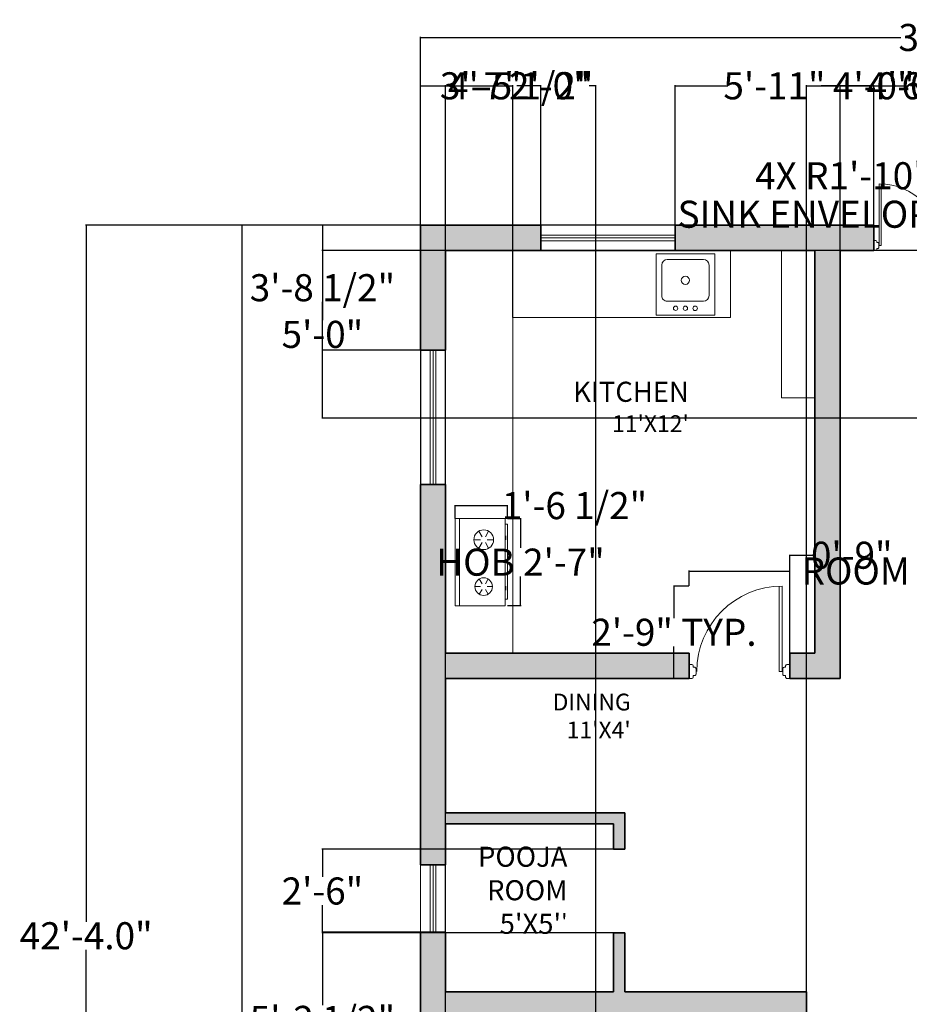
# Model space of a CAD drawing. Units: inches. Extents: x 2103 to 2702, y 2405 to 3142.
# Tile 3 of 7: x 2103 to 2421, y 2790 to 3142. Entities that reach past the tile are written whole.
import ezdxf

# ---------------------------------------------------------------- set-up
doc = ezdxf.new("R2010")
doc.units = ezdxf.units.IN
doc.linetypes.add('0', pattern=[0])
for name, color, linetype, lineweight in [('00 FURNITURE', 15, 'Continuous', 15), ('A-ANNO-DIMS', 2, 'Continuous', 18), ('A-AREA-IDEN', 7, 'Continuous', 18), ('A-EQPM', 9, 'Continuous', 18), ('A-FLOR-CASE', 8, 'Continuous', 18), ('A-FLOR-FIXT', 9, 'Continuous', 18), ('A-WALL-PATT', 8, 'Continuous', 9), ('A_TEXT_SMALL', 18, 'Continuous', 5), ('doors', 4, 'Continuous', 18), ('WALL', 7, 'Continuous', 35), ('WINDOW', 160, '0', 5), ('windows', 4, 'Continuous', 18)]:
    doc.layers.add(name, color=color, linetype=linetype, lineweight=lineweight)
doc.layers.add('FURN3D', color=229, linetype='Continuous', lineweight=5, true_color=0x4a3f41)
doc.layers.add('furniture', color=34, linetype='Continuous')
doc.styles.get("Standard").update_dxf_attribs({"font": 'arial.ttf'})
doc.dimstyles.get("Standard").update_dxf_attribs({"dimtxt": 9.68, "dimasz": 0.18, "dimexe": 0.18, "dimexo": 0.0625, "dimgap": 0.09, "dimtad": 0, "dimtih": 1, "dimtoh": 1, "dimdec": 1, "dimzin": 0, "dimdsep": 46, "dimlunit": 3, "dimtxsty": 'Standard', "dimcen": 0.09, "dimadec": 0, "dimazin": 0, "dimtfac": 1, "dimtdec": 1, "dimtofl": 0, "dimtmove": 0, "dimatfit": 3, "dimfxl": 1, "dimtolj": 1, "dimtzin": 0, "dimarcsym": 0})

# ---------------------------------------------------------------- blocks, each defined once
blk = doc.blocks.new('DDD')
at = {"layer": '00 FURNITURE'}
for p, q in [((-12579.77, -15859.53), (-12579.77, -15829.05)), ((-12578.77, -15859.53), (-12578.77, -15829.03)), ((-12612.02, -15857.03), (-12612.02, -15862.03)), ((-12611.02, -15857.03), (-12612.02, -15857.03)), ((-12610.52, -15858.03), (-12610.52, -15857.53)), ((-12577.52, -15858.03), (-12577.52, -15857.53)), ((-12577.02, -15857.03), (-12576.02, -15857.03)), ((-12576.02, -15857.03), (-12576.02, -15862.03)), ((-12610.52, -15861.53), (-12610.52, -15861.03)), ((-12578.77, -15859.53), (-12579.77, -15859.53)), ((-12577.52, -15861.53), (-12577.52, -15861.03)), ((-12612.02, -15862.03), (-12611.02, -15862.03)), ((-12576.02, -15862.03), (-12577.02, -15862.03))]:
    blk.add_line(p, q, dxfattribs=at)
for points in [[(-12610.52, -15861.03), (-12610.02, -15861.03, 0.414214), (-12609.52, -15860.53), (-12609.52, -15858.53, 0.414214), (-12610.02, -15858.03), (-12610.52, -15858.03)], [(-12577.52, -15861.03), (-12578.02, -15861.03, -0.414214), (-12578.52, -15860.53), (-12578.52, -15858.53, -0.414214), (-12578.02, -15858.03), (-12577.52, -15858.03)]]:
    blk.add_lwpolyline(points, format="xyb", dxfattribs=at)
for centre, radius, start, end in [((-12578.77, -15859.53), 30.5, 90, 180), ((-12611.02, -15857.53), 0.5, 0, 90), ((-12577.02, -15857.53), 0.5, 90, 180), ((-12611.02, -15861.53), 0.5, 270, 0), ((-12577.02, -15861.53), 0.5, 180, 270)]:
    blk.add_arc(centre, radius, start, end, dxfattribs=at)
blk = doc.blocks.new('PUJA')
at = {"layer": '00 FURNITURE'}
for p, q in [((-1941.8, -16091.75), (-1938.89, -16091.75)), ((-1941.8, -16092.33), (-1941.8, -16091.75)), ((-1941.22, -16092.62), (-1941.51, -16092.62)), ((-1939.18, -16092.62), (-1939.47, -16092.62)), ((-1938.89, -16091.75), (-1938.89, -16092.33)), ((-1940.35, -16093.35), (-1958.14, -16093.35)), ((-1940.35, -16093.93), (-1958.13, -16093.93)), ((-1940.35, -16093.35), (-1940.35, -16093.93)), ((-1940.35, -16128.93), (-1958.14, -16128.93)), ((-1940.35, -16128.35), (-1958.13, -16128.35)), ((-1941.8, -16129.96), (-1941.8, -16130.54)), ((-1941.22, -16129.66), (-1941.51, -16129.66)), ((-1940.35, -16128.93), (-1940.35, -16128.35)), ((-1939.18, -16129.66), (-1939.47, -16129.66)), ((-1938.89, -16130.54), (-1938.89, -16129.96)), ((-1941.8, -16130.54), (-1938.89, -16130.54))]:
    blk.add_line(p, q, dxfattribs=at)
for points in [[(-1939.47, -16092.62), (-1939.47, -16092.91, -0.414214), (-1939.76, -16093.21), (-1940.93, -16093.21, -0.414214), (-1941.22, -16092.91), (-1941.22, -16092.62)], [(-1939.47, -16129.66), (-1939.47, -16129.37, 0.414214), (-1939.76, -16129.08), (-1940.93, -16129.08, 0.414214), (-1941.22, -16129.37), (-1941.22, -16129.66)]]:
    blk.add_lwpolyline(points, format="xyb", dxfattribs=at)
for centre, radius, start, end in [((-1941.51, -16092.33), 0.292, 180, 270), ((-1939.18, -16092.33), 0.292, 270, 0), ((-1940.35, -16093.35), 17.79, 180, 270), ((-1940.35, -16128.93), 17.79, 90, 180), ((-1941.51, -16129.96), 0.292, 90, 180), ((-1939.18, -16129.96), 0.292, 0, 90)]:
    blk.add_arc(centre, radius, start, end, dxfattribs=at)
blk = doc.blocks.new('window')
at = {"layer": 'furniture'}
for p, q in [((1745.13, 2764.08), (1745.13, 2716.08)), ((1754.13, 2716.08), (1754.13, 2764.08))]:
    blk.add_line(p, q, dxfattribs=at)
at = {"layer": 'WINDOW'}
for p, q in [((1748.63, 2764.08), (1748.63, 2716.08)), ((1749.63, 2764.08), (1749.63, 2716.08)), ((1750.63, 2764.08), (1750.63, 2716.08))]:
    blk.add_line(p, q, dxfattribs=at)
blk = doc.blocks.new('ventilator')
at = {"layer": 'windows'}
for p, q in [((1922.12, 2523.05), (1898.12, 2523.05)), ((1922.12, 2522.05), (1898.12, 2522.05)), ((1922.12, 2521.05), (1898.12, 2521.05))]:
    blk.add_line(p, q, dxfattribs=at)
blk.add_lwpolyline([(1898.12, 2526.55), (1898.12, 2517.55), (1922.12, 2517.55), (1922.12, 2526.55)], close=True, dxfattribs=at)
blk = doc.blocks.new('A$C21540130')
at = {"layer": 'FURN3D'}
for p, q in [((1.57, 0), (1.57, 31.11)), ((9.61, 25.31), (8.63, 27.01)), ((10.79, 25.31), (11.77, 27.01)), ((9.02, 24.29, -27.54), (7.06, 24.29, -27.54)), ((9.61, 23.27), (8.63, 21.57)), ((10.79, 23.27), (11.77, 21.57)), ((11.38, 24.29, -27.54), (13.34, 24.29, -27.54)), ((9.61, 8.56), (8.43, 10.6)), ((10.79, 8.56), (11.97, 10.6)), ((9.02, 7.54), (6.67, 7.54)), ((11.38, 7.54), (13.73, 7.54)), ((9.61, 6.52), (8.43, 4.48)), ((10.79, 6.52), (11.97, 4.48))]:
    blk.add_line(p, q, dxfattribs=at)
for points in [[(0, 0), (0, 31.11), (17.9, 31.11), (17.9, 0)], [(18.68, 1.96), (18.68, 28.83), (17.9, 28.83), (17.9, 1.96)]]:
    blk.add_lwpolyline(points, close=True, dxfattribs=at)
for centre, radius in [((10.2, 24.29), 3.14), ((10.2, 7.54), 3.53)]:
    blk.add_circle(centre, radius, dxfattribs=at)
for points in [[(17.9, 24.03), (18.29, 24.03), (17.9, 25.6), (18.29, 25.6)], [(17.9, 6.05), (18.29, 6.05), (17.9, 7.62), (18.29, 7.62)]]:
    blk.add_solid(points, dxfattribs=at)
blk = doc.blocks.new('reh-flat-2')
at = {"layer": 'A_TEXT_SMALL'}
for p, q in [((486053827.2, -394630231.2), (486054182.4, -394629799.8)), ((486054182.4, -394629799.8), (486054596.6, -394630140.9)), ((486053979.5, -394630126.3), (486054157.1, -394629910.6)), ((486054228.6, -394629903.6), (486054483.5, -394630113.5)), ((486054596.6, -394630140.9), (486054241.4, -394630572.3)), ((486054241.4, -394630572.3), (486053827.2, -394630231.2)), ((486054241.3, -394630407.7), (486053986.4, -394630197.8)), ((486054490.4, -394630185), (486054312.8, -394630400.7))]:
    blk.add_line(p, q, dxfattribs=at)
for centre, radius in [((486054234.9, -394630155.7), 38.1), ((486054004.1, -394630296.2), 20.1), ((486054072.7, -394630352.7), 20.1), ((486054141.4, -394630409.3), 20.1)]:
    blk.add_circle(centre, radius, dxfattribs=at)
for centre, start, end in [((486054196.3, -394629942.9), 50.53053, 140.53053), ((486054018.7, -394630158.5), 140.53053, 230.53053), ((486054451.2, -394630152.8), 320.53053, 50.53053), ((486054273.6, -394630368.4), 230.53053, 320.53053)]:
    blk.add_arc(centre, 50.8, start, end, dxfattribs=at)
blk = doc.blocks.new('*D15')
at = {"layer": 'A-ANNO-DIMS', "color": 0, "lineweight": -2, "transparency": 16777216}
for p, q in [((2246.43, 3068.91), (2246.43, 3136.18)), ((2246.61, 3136), (2418.13, 3136)), ((2606.25, 3136), (2434.73, 3136)), ((2606.43, 3068.91), (2606.43, 3136.18))]:
    blk.add_line(p, q, dxfattribs=at)
at = {"layer": 'A-ANNO-DIMS', "color": 0, "transparency": 16777216}
for points in [[(2246.61, 3136.03), (2246.61, 3135.97), (2246.43, 3136)], [(2606.25, 3136.03), (2606.25, 3135.97), (2606.43, 3136)]]:
    blk.add_solid(points, dxfattribs=at)
at = {"layer": 'Defpoints', "color": 0, "transparency": 16777216}
for p in [(2606.43, 3136), (2246.43, 3068.85), (2606.43, 3068.85)]:
    blk.add_point(p, dxfattribs=at)
at = {"layer": 'A-ANNO-DIMS', "color": 0, "transparency": 16777216, "insert": (2426.43, 3136), "char_height": 9.68, "attachment_point": 5}
blk.add_mtext("\\A1;30'", dxfattribs=at)
blk = doc.blocks.new('*D16')
at = {"layer": 'A-ANNO-DIMS', "color": 0, "lineweight": -2, "transparency": 16777216}
for p, q in [((2246.37, 3068.85), (2182.44, 3068.85)), ((2182.62, 3068.67), (2182.62, 2762.88)), ((2182.62, 2447.03), (2182.62, 2752.81)), ((2246.37, 2446.85), (2182.44, 2446.85))]:
    blk.add_line(p, q, dxfattribs=at)
at = {"layer": 'A-ANNO-DIMS', "color": 0, "transparency": 16777216}
for points in [[(2182.59, 3068.67), (2182.65, 3068.67), (2182.62, 3068.85)], [(2182.59, 2447.03), (2182.65, 2447.03), (2182.62, 2446.85)]]:
    blk.add_solid(points, dxfattribs=at)
at = {"layer": 'Defpoints', "color": 0, "transparency": 16777216}
for p in [(2246.43, 3068.85), (2182.62, 2446.85), (2246.43, 2446.85)]:
    blk.add_point(p, dxfattribs=at)
at = {"layer": 'A-ANNO-DIMS', "color": 0, "transparency": 16777216, "insert": (2182.62, 2757.85), "char_height": 9.68, "attachment_point": 5}
blk.add_mtext('\\A1;51\'-10.0"', dxfattribs=at)
blk = doc.blocks.new('*D17')
at = {"layer": 'A-ANNO-DIMS', "color": 0, "lineweight": -2, "transparency": 16777216}
for p, q in [((2246.37, 3068.85), (2126.76, 3068.85)), ((2126.94, 3068.67), (2126.94, 2819.88)), ((2126.94, 2561.03), (2126.94, 2809.81)), ((2246.37, 2560.85), (2126.76, 2560.85))]:
    blk.add_line(p, q, dxfattribs=at)
at = {"layer": 'A-ANNO-DIMS', "color": 0, "transparency": 16777216}
for points in [[(2126.91, 3068.67), (2126.97, 3068.67), (2126.94, 3068.85)], [(2126.91, 2561.03), (2126.97, 2561.03), (2126.94, 2560.85)]]:
    blk.add_solid(points, dxfattribs=at)
at = {"layer": 'Defpoints', "color": 0, "transparency": 16777216}
for p in [(2246.43, 3068.85), (2126.94, 2560.85), (2246.43, 2560.85)]:
    blk.add_point(p, dxfattribs=at)
at = {"layer": 'A-ANNO-DIMS', "color": 0, "transparency": 16777216, "insert": (2126.94, 2814.85), "char_height": 9.68, "attachment_point": 5}
blk.add_mtext('\\A1;42\'-4.0"', dxfattribs=at)
blk = doc.blocks.new('*D22')
at = {"layer": 'A-ANNO-DIMS', "color": 0, "lineweight": -2, "transparency": 16777216}
for p, q in [((2342.43, 2939.91), (2342.43, 2945.43)), ((2342.61, 2945.25), (2378.25, 2945.25)), ((2378.43, 2939.91), (2378.43, 2945.43)), ((2378.43, 2945.25), (2378.61, 2945.25))]:
    blk.add_line(p, q, dxfattribs=at)
at = {"layer": 'A-ANNO-DIMS', "color": 0, "transparency": 16777216}
for points in [[(2342.61, 2945.28), (2342.61, 2945.22), (2342.43, 2945.25)], [(2378.25, 2945.28), (2378.25, 2945.22), (2378.43, 2945.25)]]:
    blk.add_solid(points, dxfattribs=at)
at = {"layer": 'Defpoints', "color": 0, "transparency": 16777216}
for p in [(2378.43, 2945.25), (2342.43, 2939.85), (2378.43, 2939.85)]:
    blk.add_point(p, dxfattribs=at)
at = {"layer": 'A-ANNO-DIMS', "color": 0, "transparency": 16777216, "insert": (2453.03, 2945.25), "char_height": 9.68, "attachment_point": 5}
blk.add_mtext('\\A1;ROOM DOOR 3\'-0" TYP.', dxfattribs=at)
blk = doc.blocks.new('*D23')
at = {"layer": 'A-ANNO-DIMS', "color": 0, "lineweight": -2, "transparency": 16777216}
for p, q in [((2342.37, 2939.85), (2336.85, 2939.85)), ((2337.03, 2939.67), (2337.03, 2928.38)), ((2337.03, 2907.03), (2337.03, 2918.31)), ((2342.37, 2906.85), (2336.85, 2906.85))]:
    blk.add_line(p, q, dxfattribs=at)
at = {"layer": 'A-ANNO-DIMS', "color": 0, "transparency": 16777216}
for points in [[(2337, 2939.67), (2337.06, 2939.67), (2337.03, 2939.85)], [(2337, 2907.03), (2337.06, 2907.03), (2337.03, 2906.85)]]:
    blk.add_solid(points, dxfattribs=at)
at = {"layer": 'Defpoints', "color": 0, "transparency": 16777216}
for p in [(2337.03, 2939.85), (2342.43, 2939.85), (2342.43, 2906.85)]:
    blk.add_point(p, dxfattribs=at)
at = {"layer": 'A-ANNO-DIMS', "color": 0, "transparency": 16777216, "insert": (2337.03, 2923.35), "char_height": 9.68, "attachment_point": 5}
blk.add_mtext('\\A1;2\'-9" TYP.', dxfattribs=at)
blk = doc.blocks.new('*D32')
at = {"layer": 'A-ANNO-DIMS', "color": 0, "lineweight": -2, "transparency": 16777216}
for p, q in [((2523.7, 3069.82), (2527.3, 3072.78)), ((2527.05, 3072.8), (2526.87, 3072.8)), ((2527.16, 3072.66), (2527.05, 3072.8)), ((2546.29, 3049.43), (2527.27, 3072.52)), ((2542.95, 3046.44), (2546.55, 3049.4))]:
    blk.add_line(p, q, dxfattribs=at)
at = {"layer": 'A-ANNO-DIMS', "color": 0, "transparency": 16777216}
for points in [[(2527.3, 3072.54), (2527.25, 3072.51), (2527.16, 3072.66)], [(2546.31, 3049.45), (2546.27, 3049.41), (2546.41, 3049.29)]]:
    blk.add_solid(points, dxfattribs=at)
at = {"layer": 'Defpoints', "color": 0, "transparency": 16777216}
for p in [(2523.65, 3069.78), (2527.16, 3072.66), (2542.9, 3046.4)]:
    blk.add_point(p, dxfattribs=at)
at = {"layer": 'A-ANNO-DIMS', "color": 0, "transparency": 16777216, "insert": (2430.03, 3072.8), "char_height": 9.68, "attachment_point": 5}
blk.add_mtext('\\A1;SINK ENVELOPE 2\'-6 1/2" TYP.', dxfattribs=at)
blk = doc.blocks.new('*D34')
at = {"layer": 'A-ANNO-DIMS', "color": 0, "lineweight": -2, "transparency": 16777216}
for p, q in [((2277.58, 2963.97), (2282.36, 2963.97)), ((2282.18, 2963.79), (2282.18, 2953.52)), ((2282.18, 2933.05), (2282.18, 2943.32)), ((2277.58, 2932.87), (2282.36, 2932.87))]:
    blk.add_line(p, q, dxfattribs=at)
at = {"layer": 'A-ANNO-DIMS', "color": 0, "transparency": 16777216}
for points in [[(2282.15, 2963.79), (2282.21, 2963.79), (2282.18, 2963.97)], [(2282.15, 2933.05), (2282.21, 2933.05), (2282.18, 2932.87)]]:
    blk.add_solid(points, dxfattribs=at)
at = {"layer": 'Defpoints', "color": 0, "transparency": 16777216}
for p in [(2277.52, 2963.97), (2277.52, 2932.87), (2282.18, 2932.87)]:
    blk.add_point(p, dxfattribs=at)
at = {"layer": 'A-ANNO-DIMS', "color": 0, "transparency": 16777216, "insert": (2282.18, 2948.42), "char_height": 9.68, "attachment_point": 5}
blk.add_mtext('\\A1;HOB 2\'-7"', dxfattribs=at)
blk = doc.blocks.new('*D35')
at = {"layer": 'A-ANNO-DIMS', "color": 0, "lineweight": -2, "transparency": 16777216}
for p, q in [((2258.83, 2964.03), (2258.83, 2968.82)), ((2259.01, 2968.64), (2277.34, 2968.64)), ((2277.52, 2964.03), (2277.52, 2968.82)), ((2277.52, 2968.64), (2277.7, 2968.64))]:
    blk.add_line(p, q, dxfattribs=at)
at = {"layer": 'A-ANNO-DIMS', "color": 0, "transparency": 16777216}
for points in [[(2259.01, 2968.67), (2259.01, 2968.61), (2258.83, 2968.64)], [(2277.34, 2968.67), (2277.34, 2968.61), (2277.52, 2968.64)]]:
    blk.add_solid(points, dxfattribs=at)
at = {"layer": 'Defpoints', "color": 0, "transparency": 16777216}
for p in [(2277.52, 2968.64), (2258.83, 2963.97), (2277.52, 2963.97)]:
    blk.add_point(p, dxfattribs=at)
at = {"layer": 'A-ANNO-DIMS', "color": 0, "transparency": 16777216, "insert": (2301.47, 2968.64), "char_height": 9.68, "attachment_point": 5}
blk.add_mtext('\\A1;1\'-6 1/2"', dxfattribs=at)
blk = doc.blocks.new('*D40')
at = {"layer": 'A-ANNO-DIMS', "color": 0, "lineweight": -2, "transparency": 16777216}
for p, q in [((2396.43, 2906.91), (2396.43, 3118.9)), ((2444.43, 2842.91), (2444.43, 3118.9)), ((2396.61, 3118.72), (2407.28, 3118.72)), ((2444.25, 3118.72), (2433.58, 3118.72))]:
    blk.add_line(p, q, dxfattribs=at)
at = {"layer": 'A-ANNO-DIMS', "color": 0, "transparency": 16777216}
for points in [[(2396.61, 3118.75), (2396.61, 3118.69), (2396.43, 3118.72)], [(2444.25, 3118.75), (2444.25, 3118.69), (2444.43, 3118.72)]]:
    blk.add_solid(points, dxfattribs=at)
at = {"layer": 'Defpoints', "color": 0, "transparency": 16777216}
for p in [(2444.43, 3118.72), (2396.43, 2906.85), (2444.43, 2842.85)]:
    blk.add_point(p, dxfattribs=at)
at = {"layer": 'A-ANNO-DIMS', "color": 0, "transparency": 16777216, "insert": (2420.43, 3118.72), "char_height": 9.68, "attachment_point": 5}
blk.add_mtext('\\A1;4\'-0"', dxfattribs=at)
blk = doc.blocks.new('*D48')
at = {"layer": 'A-ANNO-DIMS', "color": 0, "lineweight": -2, "transparency": 16777216}
for p, q in [((2255.43, 2569.91), (2255.43, 3118.9)), ((2309.13, 2569.91), (2309.13, 3118.9)), ((2255.61, 3118.72), (2257.85, 3118.72)), ((2308.95, 3118.72), (2306.71, 3118.72))]:
    blk.add_line(p, q, dxfattribs=at)
at = {"layer": 'A-ANNO-DIMS', "color": 0, "transparency": 16777216}
for points in [[(2255.61, 3118.75), (2255.61, 3118.69), (2255.43, 3118.72)], [(2308.95, 3118.75), (2308.95, 3118.69), (2309.13, 3118.72)]]:
    blk.add_solid(points, dxfattribs=at)
at = {"layer": 'Defpoints', "color": 0, "transparency": 16777216}
for p in [(2309.13, 3118.72), (2255.43, 2569.85), (2309.13, 2569.85)]:
    blk.add_point(p, dxfattribs=at)
at = {"layer": 'A-ANNO-DIMS', "color": 0, "transparency": 16777216, "insert": (2282.28, 3118.72), "char_height": 9.68, "attachment_point": 5}
blk.add_mtext('\\A1;4\'-5 1/2"', dxfattribs=at)
blk = doc.blocks.new('*D53')
at = {"layer": 'A-ANNO-DIMS', "color": 0, "lineweight": -2, "transparency": 16777216}
for p, q in [((2246.37, 2816.19), (2211.2, 2816.19)), ((2211.38, 2816.01), (2211.38, 2790.04)), ((2211.38, 2753.88), (2211.38, 2779.85)), ((2246.37, 2753.7), (2211.2, 2753.7))]:
    blk.add_line(p, q, dxfattribs=at)
at = {"layer": 'A-ANNO-DIMS', "color": 0, "transparency": 16777216}
for points in [[(2211.35, 2816.01), (2211.41, 2816.01), (2211.38, 2816.19)], [(2211.35, 2753.88), (2211.41, 2753.88), (2211.38, 2753.7)]]:
    blk.add_solid(points, dxfattribs=at)
at = {"layer": 'Defpoints', "color": 0, "transparency": 16777216}
for p in [(2211.38, 2816.19), (2246.43, 2816.19), (2246.43, 2753.7)]:
    blk.add_point(p, dxfattribs=at)
at = {"layer": 'A-ANNO-DIMS', "color": 0, "transparency": 16777216, "insert": (2211.38, 2784.95), "char_height": 9.68, "attachment_point": 5}
blk.add_mtext('\\A1;5\'-2 1/2"', dxfattribs=at)
blk = doc.blocks.new('*D54')
at = {"layer": 'A-ANNO-DIMS', "color": 0, "lineweight": -2, "transparency": 16777216}
for p, q in [((2246.37, 3068.85), (2211.2, 3068.85)), ((2211.38, 3068.67), (2211.38, 3051.63)), ((2211.38, 3024.41), (2211.38, 3041.44)), ((2246.37, 3024.23), (2211.2, 3024.23))]:
    blk.add_line(p, q, dxfattribs=at)
at = {"layer": 'A-ANNO-DIMS', "color": 0, "transparency": 16777216}
for points in [[(2211.35, 3068.67), (2211.41, 3068.67), (2211.38, 3068.85)], [(2211.35, 3024.41), (2211.41, 3024.41), (2211.38, 3024.23)]]:
    blk.add_solid(points, dxfattribs=at)
at = {"layer": 'Defpoints', "color": 0, "transparency": 16777216}
for p in [(2211.38, 3068.85), (2246.43, 3068.85), (2246.43, 3024.23)]:
    blk.add_point(p, dxfattribs=at)
at = {"layer": 'A-ANNO-DIMS', "color": 0, "transparency": 16777216, "insert": (2211.38, 3046.54), "char_height": 9.68, "attachment_point": 5}
blk.add_mtext('\\A1;3\'-8 1/2"', dxfattribs=at)
blk = doc.blocks.new('*D55')
at = {"layer": 'A-ANNO-DIMS', "color": 0, "lineweight": -2, "transparency": 16777216}
for p, q in [((2246.43, 3068.91), (2246.43, 3118.9)), ((2289.47, 3068.91), (2289.47, 3118.9)), ((2246.61, 3118.72), (2255, 3118.72)), ((2289.29, 3118.72), (2280.9, 3118.72))]:
    blk.add_line(p, q, dxfattribs=at)
at = {"layer": 'A-ANNO-DIMS', "color": 0, "transparency": 16777216}
for points in [[(2246.61, 3118.75), (2246.61, 3118.69), (2246.43, 3118.72)], [(2289.29, 3118.75), (2289.29, 3118.69), (2289.47, 3118.72)]]:
    blk.add_solid(points, dxfattribs=at)
at = {"layer": 'Defpoints', "color": 0, "transparency": 16777216}
for p in [(2289.47, 3118.72), (2246.43, 3068.85), (2289.47, 3068.85)]:
    blk.add_point(p, dxfattribs=at)
at = {"layer": 'A-ANNO-DIMS', "color": 0, "transparency": 16777216, "insert": (2267.95, 3118.72), "char_height": 9.68, "attachment_point": 5}
blk.add_mtext('\\A1;3\'-7"', dxfattribs=at)
blk = doc.blocks.new('*D56')
at = {"layer": 'A-ANNO-DIMS', "color": 0, "lineweight": -2, "transparency": 16777216}
for p, q in [((2337.47, 3068.91), (2337.47, 3118.9)), ((2408.43, 3068.91), (2408.43, 3118.9)), ((2337.65, 3118.72), (2356.23, 3118.72)), ((2408.25, 3118.72), (2389.67, 3118.72))]:
    blk.add_line(p, q, dxfattribs=at)
at = {"layer": 'A-ANNO-DIMS', "color": 0, "transparency": 16777216}
for points in [[(2337.65, 3118.75), (2337.65, 3118.69), (2337.47, 3118.72)], [(2408.25, 3118.75), (2408.25, 3118.69), (2408.43, 3118.72)]]:
    blk.add_solid(points, dxfattribs=at)
at = {"layer": 'Defpoints', "color": 0, "transparency": 16777216}
for p in [(2408.43, 3118.72), (2337.47, 3068.85), (2408.43, 3068.85)]:
    blk.add_point(p, dxfattribs=at)
at = {"layer": 'A-ANNO-DIMS', "color": 0, "transparency": 16777216, "insert": (2372.95, 3118.72), "char_height": 9.68, "attachment_point": 5}
blk.add_mtext('\\A1;5\'-11"', dxfattribs=at)
blk = doc.blocks.new('*D63')
at = {"layer": 'A-ANNO-DIMS', "color": 0, "lineweight": -2, "transparency": 16777216}
for p, q in [((2255.43, 3059.91), (2255.43, 3118.9)), ((2279.43, 3035.91), (2279.43, 3118.9)), ((2255.61, 3118.72), (2279.25, 3118.72)), ((2279.43, 3118.72), (2279.61, 3118.72))]:
    blk.add_line(p, q, dxfattribs=at)
at = {"layer": 'A-ANNO-DIMS', "color": 0, "transparency": 16777216}
for points in [[(2255.61, 3118.75), (2255.61, 3118.69), (2255.43, 3118.72)], [(2279.25, 3118.75), (2279.25, 3118.69), (2279.43, 3118.72)]]:
    blk.add_solid(points, dxfattribs=at)
at = {"layer": 'Defpoints', "color": 0, "transparency": 16777216}
for p in [(2279.43, 3118.72), (2255.43, 3059.85), (2279.43, 3035.85)]:
    blk.add_point(p, dxfattribs=at)
at = {"layer": 'A-ANNO-DIMS', "color": 0, "transparency": 16777216, "insert": (2292.65, 3118.72), "char_height": 9.68, "attachment_point": 5}
blk.add_mtext('\\A1;2\'-0"', dxfattribs=at)
blk = doc.blocks.new('*D64')
at = {"layer": 'A-ANNO-DIMS', "color": 0, "lineweight": -2, "transparency": 16777216}
for p, q in [((2396.43, 3059.91), (2396.43, 3118.9)), ((2469.43, 3059.91), (2469.43, 3118.9)), ((2396.61, 3118.72), (2419.95, 3118.72)), ((2469.25, 3118.72), (2445.91, 3118.72))]:
    blk.add_line(p, q, dxfattribs=at)
at = {"layer": 'A-ANNO-DIMS', "color": 0, "transparency": 16777216}
for points in [[(2396.61, 3118.75), (2396.61, 3118.69), (2396.43, 3118.72)], [(2469.25, 3118.75), (2469.25, 3118.69), (2469.43, 3118.72)]]:
    blk.add_solid(points, dxfattribs=at)
at = {"layer": 'Defpoints', "color": 0, "transparency": 16777216}
for p in [(2469.43, 3118.72), (2396.43, 3059.85), (2469.43, 3059.85)]:
    blk.add_point(p, dxfattribs=at)
at = {"layer": 'A-ANNO-DIMS', "color": 0, "transparency": 16777216, "insert": (2432.93, 3118.72), "char_height": 9.68, "attachment_point": 5}
blk.add_mtext('\\A1;6\'-1"', dxfattribs=at)
blk = doc.blocks.new('*D65')
at = {"layer": 'A-ANNO-DIMS', "color": 0, "lineweight": -2, "transparency": 16777216}
for p, q in [((2315.37, 2845.85), (2211.2, 2845.85)), ((2211.38, 2845.67), (2211.38, 2835.88)), ((2211.38, 2816.03), (2211.38, 2825.81)), ((2315.37, 2815.85), (2211.2, 2815.85))]:
    blk.add_line(p, q, dxfattribs=at)
at = {"layer": 'A-ANNO-DIMS', "color": 0, "transparency": 16777216}
for points in [[(2211.35, 2845.67), (2211.41, 2845.67), (2211.38, 2845.85)], [(2211.35, 2816.03), (2211.41, 2816.03), (2211.38, 2815.85)]]:
    blk.add_solid(points, dxfattribs=at)
at = {"layer": 'Defpoints', "color": 0, "transparency": 16777216}
for p in [(2315.43, 2845.85), (2211.38, 2815.85), (2315.43, 2815.85)]:
    blk.add_point(p, dxfattribs=at)
at = {"layer": 'A-ANNO-DIMS', "color": 0, "transparency": 16777216, "insert": (2211.38, 2830.85), "char_height": 9.68, "attachment_point": 5}
blk.add_mtext('\\A1;2\'-6"', dxfattribs=at)
blk = doc.blocks.new('*D66')
at = {"layer": 'A-ANNO-DIMS', "color": 0, "lineweight": -2, "transparency": 16777216}
for p, q in [((2384.43, 2794.91), (2384.43, 3118.9)), ((2432.43, 2794.91), (2432.43, 3118.9)), ((2384.61, 3118.72), (2395.28, 3118.72)), ((2432.25, 3118.72), (2421.58, 3118.72))]:
    blk.add_line(p, q, dxfattribs=at)
at = {"layer": 'A-ANNO-DIMS', "color": 0, "transparency": 16777216}
for points in [[(2384.61, 3118.75), (2384.61, 3118.69), (2384.43, 3118.72)], [(2432.25, 3118.75), (2432.25, 3118.69), (2432.43, 3118.72)]]:
    blk.add_solid(points, dxfattribs=at)
at = {"layer": 'Defpoints', "color": 0, "transparency": 16777216}
for p in [(2384.43, 3118.72), (2384.43, 2794.85), (2432.43, 2794.85)]:
    blk.add_point(p, dxfattribs=at)
at = {"layer": 'A-ANNO-DIMS', "color": 0, "transparency": 16777216, "insert": (2408.43, 3118.72), "char_height": 9.68, "attachment_point": 5}
blk.add_mtext('\\A1;4\'-0"', dxfattribs=at)
blk = doc.blocks.new('*D68')
at = {"layer": 'A-ANNO-DIMS', "color": 0, "lineweight": -2, "transparency": 16777216}
for p, q in [((2469.37, 3059.85), (2211.2, 3059.85)), ((2211.38, 3059.67), (2211.38, 3034.88)), ((2211.38, 3000.03), (2211.38, 3024.81)), ((2469.37, 2999.85), (2211.2, 2999.85))]:
    blk.add_line(p, q, dxfattribs=at)
at = {"layer": 'A-ANNO-DIMS', "color": 0, "transparency": 16777216}
for points in [[(2211.35, 3059.67), (2211.41, 3059.67), (2211.38, 3059.85)], [(2211.35, 3000.03), (2211.41, 3000.03), (2211.38, 2999.85)]]:
    blk.add_solid(points, dxfattribs=at)
at = {"layer": 'Defpoints', "color": 0, "transparency": 16777216}
for p in [(2469.43, 3059.85), (2211.38, 2999.85), (2469.43, 2999.85)]:
    blk.add_point(p, dxfattribs=at)
at = {"layer": 'A-ANNO-DIMS', "color": 0, "transparency": 16777216, "insert": (2211.38, 3029.85), "char_height": 9.68, "attachment_point": 5}
blk.add_mtext('\\A1;5\'-0"', dxfattribs=at)
blk = doc.blocks.new('*D74')
at = {"layer": 'A-ANNO-DIMS', "color": 0, "lineweight": -2, "transparency": 16777216}
for p, q in [((2378.43, 2915.91), (2378.43, 2951.08)), ((2378.61, 2950.9), (2387.25, 2950.9)), ((2387.43, 2915.91), (2387.43, 2951.08)), ((2387.43, 2950.9), (2387.61, 2950.9))]:
    blk.add_line(p, q, dxfattribs=at)
at = {"layer": 'A-ANNO-DIMS', "color": 0, "transparency": 16777216}
for points in [[(2378.61, 2950.93), (2378.61, 2950.87), (2378.43, 2950.9)], [(2387.25, 2950.93), (2387.25, 2950.87), (2387.43, 2950.9)]]:
    blk.add_solid(points, dxfattribs=at)
at = {"layer": 'Defpoints', "color": 0, "transparency": 16777216}
for p in [(2387.43, 2950.9), (2378.43, 2915.85), (2387.43, 2915.85)]:
    blk.add_point(p, dxfattribs=at)
at = {"layer": 'A-ANNO-DIMS', "color": 0, "transparency": 16777216, "insert": (2400.57, 2950.9), "char_height": 9.68, "attachment_point": 5}
blk.add_mtext('\\A1;0\'-9"', dxfattribs=at)
blk = doc.blocks.new('*D81')
at = {"layer": 'A-ANNO-DIMS', "color": 0, "lineweight": -2, "transparency": 16777216}
for p, q in [((2429.36, 3086.56), (2429.54, 3086.56)), ((2429.54, 3086.56), (2438.75, 3077.34)), ((2454.36, 3061.65), (2454.54, 3061.65)), ((2454.45, 3061.56), (2454.45, 3061.74))]:
    blk.add_line(p, q, dxfattribs=at)
at = {"layer": 'A-ANNO-DIMS', "color": 0, "transparency": 16777216}
blk.add_solid([(2438.77, 3077.37), (2438.73, 3077.32), (2438.88, 3077.22)], dxfattribs=at)
at = {"layer": 'Defpoints', "color": 0, "transparency": 16777216}
for p in [(2438.88, 3077.22), (2454.45, 3061.65)]:
    blk.add_point(p, dxfattribs=at)
at = {"layer": 'A-ANNO-DIMS', "color": 0, "transparency": 16777216, "insert": (2397.41, 3086.56), "char_height": 9.68, "attachment_point": 5}
blk.add_mtext('\\A1;4X R1\'-10"', dxfattribs=at)

msp = doc.modelspace()

# ---------------------------------------------------------------- hatches: boundary and pattern name
at = {"layer": 'A-WALL-PATT'}
h = msp.add_hatch(color=256, dxfattribs=at)
h.dxf.hatch_style = 1
h.paths.add_polyline_path([(2255.43, 3059.85), (2289.47, 3059.85), (2289.47, 3068.85), (2289.47, 3068.85), (2246.43, 3068.85), (2246.43, 3024.23), (2255.43, 3024.23)])
h.paths.add_polyline_path([(2408.43, 3068.85), (2337.47, 3068.85), (2337.47, 3059.85), (2387.43, 3059.85), (2387.43, 3035.85), (2387.43, 2915.85), (2378.43, 2915.85), (2378.43, 2906.85), (2396.43, 2906.85), (2396.43, 3059.85), (2408.43, 3059.85), (2408.43, 3063.45)])
h.paths.add_polyline_path([(2482.43, 3068.85), (2456.43, 3068.85), (2456.43, 3059.85), (2469.43, 3059.85), (2469.43, 2999.85), (2473.43, 2999.85), (2473.43, 3003.85), (2473.43, 3059.85), (2482.43, 3059.85)])
h.paths.add_polyline_path([(2606.43, 3068.85), (2506.43, 3068.85), (2506.43, 3059.85), (2533.43, 3059.85), (2533.43, 3045.85), (2533.77, 3045.85, -0.143035), (2534.31, 3046), (2537.43, 3046), (2537.43, 3059.85), (2597.43, 3059.85), (2597.43, 3043.85), (2606.43, 3043.85)])
h = msp.add_hatch(color=256, dxfattribs=at)
h.dxf.hatch_style = 1
h.paths.add_polyline_path([(2342.43, 2911.85), (2342.43, 2915.85), (2255.43, 2915.85), (2255.43, 2976.23), (2246.43, 2976.23), (2246.43, 2840.19), (2255.43, 2840.19), (2255.43, 2854.85), (2315.43, 2854.85), (2315.43, 2845.85), (2319.43, 2845.85), (2319.43, 2858.85), (2255.43, 2858.85), (2255.43, 2906.85), (2342.43, 2906.85)])
h.paths.add_polyline_path([(2384.43, 2794.85), (2319.43, 2794.85), (2319.43, 2815.85), (2315.43, 2815.85), (2315.43, 2794.85), (2255.43, 2794.85), (2255.43, 2816.19), (2246.43, 2816.19), (2246.43, 2753.7), (2255.43, 2753.7), (2255.43, 2785.85), (2384.43, 2785.85)])
h.paths.add_polyline_path([(2606.43, 2963.85), (2597.43, 2963.85), (2597.43, 2951.85), (2537.43, 2951.85), (2537.43, 2957.85), (2533.43, 2957.85), (2533.43, 2951.85), (2469.43, 2951.85), (2444.43, 2951.85), (2444.43, 2842.85), (2449.43, 2842.85), (2453.43, 2842.85), (2453.43, 2942.85), (2597.43, 2942.85), (2597.43, 2904.89), (2606.43, 2904.89)])
h.paths.add_polyline_path([(2606.43, 3019.85), (2597.43, 3019.85), (2597.43, 3003.85), (2537.43, 3003.85), (2537.43, 3015.85), (2533.43, 3015.85), (2533.43, 2987.85), (2537.43, 2987.85), (2537.43, 2999.85), (2597.43, 2999.85), (2597.43, 2987.85), (2606.43, 2987.85)])
h.paths.add_polyline_path([(2606.43, 2856.89), (2597.43, 2856.89), (2597.43, 2774.85), (2552.43, 2774.85), (2552.43, 2765.85), (2597.43, 2765.85), (2597.43, 2749.52), (2606.43, 2749.52)])
h.paths.add_polyline_path([(2522.43, 2774.85), (2453.43, 2774.85), (2453.43, 2806.85), (2444.43, 2806.85), (2444.43, 2794.85), (2432.43, 2794.85), (2432.43, 2785.85), (2444.43, 2785.85), (2444.43, 2765.85), (2453.43, 2765.85), (2509.43, 2765.85), (2509.43, 2705.85), (2498.43, 2705.85), (2498.43, 2701.85), (2597.43, 2701.85), (2597.43, 2678.29), (2606.43, 2678.29), (2606.43, 2725.52), (2597.43, 2725.52), (2597.43, 2705.85), (2513.43, 2705.85), (2513.43, 2765.85), (2522.43, 2765.85)])
h.paths.add_polyline_path([(2255.43, 2705.7), (2246.43, 2705.7), (2246.43, 2646.55), (2255.43, 2646.55)])
h.paths.add_polyline_path([(2255.43, 2598.55), (2246.43, 2598.55), (2246.43, 2560.85), (2309.13, 2560.85), (2309.13, 2569.85), (2309.13, 2569.85), (2255.43, 2569.85)])
h.paths.add_polyline_path([(2495.43, 2569.85), (2495.43, 2569.85), (2453.43, 2569.85), (2453.43, 2701.85), (2462.43, 2701.85), (2462.43, 2705.85), (2444.43, 2705.85), (2444.43, 2569.85), (2432.43, 2569.85), (2432.43, 2564.45), (2432.43, 2564.45), (2432.43, 2560.85), (2495.43, 2560.85)])
h.paths.add_polyline_path([(2384.43, 2569.85), (2357.13, 2569.85), (2357.13, 2560.85), (2384.43, 2560.85)])
h.paths.add_polyline_path([(2606.43, 2630.29), (2597.43, 2630.29), (2597.43, 2569.85), (2543.43, 2569.85), (2543.43, 2560.85), (2597.43, 2560.85), (2597.43, 2455.85), (2450.43, 2455.85), (2450.43, 2446.85), (2606.43, 2446.85)])

# ---------------------------------------------------------------- linework, layer by layer
at = {"layer": 'A-FLOR-CASE'}
for p, q in [((2357.24, 3035.85), (2357.24, 3059.85)), ((2387.43, 3059.85), (2375.43, 3059.85)), ((2375.43, 3059.85), (2375.43, 3007.19)), ((2387.43, 3059.85), (2387.43, 3035.85)), ((2279.43, 2915.85), (2279.43, 3035.85)), ((2357.24, 3035.85), (2279.43, 3035.85)), ((2375.43, 3007.19), (2387.43, 3007.19)), ((2255.43, 2915.85), (2279.43, 2915.85))]:
    msp.add_line(p, q, dxfattribs=at)
at = {"layer": 'WALL'}
for p, q in [((2246.43, 3068.85), (2289.47, 3068.85)), ((2246.43, 3068.85), (2246.43, 3024.23)), ((2289.47, 3059.85), (2289.47, 3068.85)), ((2337.47, 3059.85), (2337.47, 3068.85)), ((2337.47, 3068.85), (2408.43, 3068.85)), ((2408.43, 3068.85), (2408.43, 3059.85)), ((2255.43, 3059.85), (2255.43, 3024.23)), ((2255.43, 3059.85), (2289.47, 3059.85)), ((2337.47, 3059.85), (2387.43, 3059.85)), ((2387.43, 3059.85), (2387.43, 2915.85)), ((2396.43, 3059.85), (2396.43, 2906.85)), ((2396.43, 3059.85), (2408.43, 3059.85)), ((2255.43, 3024.23), (2246.43, 3024.23)), ((2255.43, 2976.23), (2246.43, 2976.23)), ((2246.43, 2976.23), (2246.43, 2840.19)), ((2255.43, 2976.23), (2255.43, 2915.85)), ((2255.43, 2915.85), (2342.43, 2915.85)), ((2342.43, 2915.85), (2342.43, 2906.85)), ((2378.43, 2915.85), (2378.43, 2906.85)), ((2378.43, 2915.85), (2387.43, 2915.85)), ((2255.43, 2906.85), (2342.43, 2906.85)), ((2255.43, 2906.85), (2255.43, 2858.85)), ((2378.43, 2906.85), (2396.43, 2906.85)), ((2255.43, 2858.85), (2319.43, 2858.85)), ((2319.43, 2858.85), (2319.43, 2845.85)), ((2255.43, 2854.85), (2315.43, 2854.85)), ((2255.43, 2854.85), (2255.43, 2840.19)), ((2315.43, 2854.85), (2315.43, 2845.85)), ((2315.43, 2845.85), (2319.43, 2845.85)), ((2255.43, 2840.19), (2246.43, 2840.19)), ((2255.43, 2816.19), (2246.43, 2816.19)), ((2246.43, 2816.19), (2246.43, 2753.7)), ((2255.43, 2816.19), (2255.43, 2794.85)), ((2315.43, 2815.85), (2319.43, 2815.85)), ((2315.43, 2815.85), (2315.43, 2794.85)), ((2319.43, 2815.85), (2319.43, 2794.85)), ((2255.43, 2794.85), (2315.43, 2794.85)), ((2319.43, 2794.85), (2384.43, 2794.85)), ((2384.43, 2794.85), (2384.43, 2785.85))]:
    msp.add_line(p, q, dxfattribs=at)

# ---------------------------------------------------------------- block references
at = {"layer": 'A-EQPM', "xscale": -1, "rotation": 180}
msp.add_blockref('A$C21540130', (2258.83, 2963.97), dxfattribs=at)
at = {"layer": 'A-FLOR-FIXT', "xscale": 0.0391972730482577, "yscale": 0.0391972730482577, "zscale": 0.0391972730482577, "rotation": 39.46947596224971}
msp.add_blockref('reh-flat-2', (-24537873.62, -166622.04), dxfattribs=at)
at = {"layer": 'doors', "xscale": 1.237379162154587, "yscale": 1.237379162154587, "zscale": 1.237379162154587, "rotation": 270.0000000034012}
msp.add_blockref('PUJA', (22368.02, 660.71), dxfattribs=at)
at = {"layer": 'doors', "rotation": 359.9999999934867}
msp.add_blockref('DDD', (14954.45, 18768.87), dxfattribs=at)
at = {"layer": 'windows'}
for name, p, rotation in [('window', (-426.61, 4813.97), 270), ('window', (4000.56, 5740.3), 180), ('ventilator', (-271.12, 4738.32), 270)]:
    msp.add_blockref(name, p, dxfattribs=dict(at, rotation=rotation))

# ---------------------------------------------------------------- texts
at = {"layer": 'A-AREA-IDEN', "char_height": 7.1875, "attachment_point": 3}
for s, insert in [("KITCHEN{\\H0.83478x;  11'X12'}", (2342.34, 3012.92)), (" {\\H0.83478x;DINING \\P11'X4'}", (2321.57, 2901.41)), ("POOJA ROOM\\P5'X5'{\\H0.83478x;'}", (2298.97, 2846.7))]:
    msp.add_mtext_dynamic_manual_height_columns(s, width=41.3807, gutter_width=12.5, heights=[0], dxfattribs=dict(at, insert=insert))

# ---------------------------------------------------------------- dimensions: what is measured, and where the dimension line sits
at = {"layer": 'A-ANNO-DIMS'}
for base, p1, p2, override, picture, middle in [((2606.43, 3136), (2246.43, 3068.85), (2606.43, 3068.85), {"dimclrd": 0, "dimclre": 0, "dimclrt": 0}, '*D15', (2426.43, 3136)), ((2309.13, 3118.72), (2255.43, 2569.85), (2309.13, 2569.85), {"dimdec": 1, "dimlfac": 1, "dimrnd": 0, "dimzin": 1, "dimdsep": 46, "dimlunit": 4, "dimfrac": 2}, '*D48', (2282.28, 3118.72)), ((2289.47, 3118.72), (2246.43, 3068.85), (2289.47, 3068.85), {"dimdec": 1, "dimlfac": 1, "dimrnd": 0, "dimzin": 1, "dimdsep": 46, "dimlunit": 4, "dimfrac": 2}, '*D55', (2267.95, 3118.72)), ((2279.43, 3118.72), (2255.43, 3059.85), (2279.43, 3035.85), {"dimdec": 1, "dimlfac": 1, "dimrnd": 0, "dimzin": 1, "dimdsep": 46, "dimlunit": 4, "dimfrac": 2}, '*D63', (2292.65, 3118.72)), ((2408.43, 3118.72), (2337.47, 3068.85), (2408.43, 3068.85), {"dimdec": 1, "dimlfac": 1, "dimrnd": 0, "dimzin": 1, "dimdsep": 46, "dimlunit": 4, "dimfrac": 2}, '*D56', (2372.95, 3118.72)), ((2384.43, 3118.72), (2432.43, 2794.85), (2384.43, 2794.85), {"dimdec": 1, "dimlfac": 1, "dimrnd": 0, "dimzin": 1, "dimdsep": 46, "dimlunit": 4, "dimfrac": 2}, '*D66', (2408.43, 3118.72)), ((2444.43, 3118.72), (2396.43, 2906.85), (2444.43, 2842.85), {"dimdec": 1, "dimlfac": 1, "dimrnd": 0, "dimzin": 1, "dimdsep": 46, "dimlunit": 4, "dimfrac": 2}, '*D40', (2420.43, 3118.72)), ((2469.43, 3118.72), (2396.43, 3059.85), (2469.43, 3059.85), {"dimdec": 1, "dimlfac": 1, "dimrnd": 0, "dimzin": 1, "dimdsep": 46, "dimlunit": 4, "dimfrac": 2}, '*D64', (2432.93, 3118.72)), ((2277.52, 2968.64), (2258.83, 2963.97), (2277.52, 2963.97), {"dimdec": 1, "dimlfac": 1, "dimrnd": 0, "dimzin": 1, "dimdsep": 46, "dimlunit": 4, "dimfrac": 2}, '*D35', (2301.47, 2968.64))]:
    dim = msp.add_linear_dim(base=base, p1=p1, p2=p2, dimstyle='Standard', override=override, dxfattribs=at)
    dim.commit()
    dim.dimension.update_dxf_attribs({"geometry": picture, "text_midpoint": middle})
for base, p1, p2, angle, text, picture, middle in [((2527.16, 3072.66), (2542.9, 3046.4), (2523.65, 3069.78), 129.4695, 'SINK ENVELOPE <> TYP.', '*D32', (2430.03, 3072.8)), ((2378.43, 2945.25), (2342.43, 2939.85), (2378.43, 2939.85), 360, 'ROOM DOOR <> TYP.', '*D22', (2453.03, 2945.25)), ((2282.18, 2932.87), (2277.52, 2963.97), (2277.52, 2932.87), 270, 'HOB <>', '*D34', (2282.18, 2948.42)), ((2337.03, 2939.85), (2342.43, 2906.85), (2342.43, 2939.85), 90, '<> TYP.', '*D23', (2337.03, 2923.35))]:
    dim = msp.add_linear_dim(base=base, p1=p1, p2=p2, angle=angle, text=text, dimstyle='Standard', override={"dimdec": 1, "dimlfac": 1, "dimrnd": 0, "dimzin": 1, "dimdsep": 46, "dimlunit": 4, "dimfrac": 2}, dxfattribs=at)
    dim.commit()
    dim.dimension.update_dxf_attribs({"geometry": picture, "text_midpoint": middle})
dim = msp.add_radius_dim(center=(2454.45, 3061.65), mpoint=(2438.88, 3077.22), text='4X <>', dimstyle='Standard', override={"dimdec": 1, "dimlfac": 1, "dimrnd": 0, "dimzin": 1, "dimdsep": 46, "dimlunit": 4, "dimfrac": 2}, dxfattribs=at)
dim.commit()
dim.dimension.update_dxf_attribs({"geometry": '*D81', "text_midpoint": (2397.41, 3086.56), "dimtype": 164})
for base, p1, p2, angle, override, picture, middle in [((2126.94, 2560.85), (2246.43, 3068.85), (2246.43, 2560.85), 90, {"dimclrd": 0, "dimclre": 0, "dimclrt": 0}, '*D17', (2126.94, 2814.85)), ((2182.62, 2446.85), (2246.43, 3068.85), (2246.43, 2446.85), 90, {"dimclrd": 0, "dimclre": 0, "dimclrt": 0}, '*D16', (2182.62, 2757.85)), ((2211.38, 3068.85), (2246.43, 3024.23), (2246.43, 3068.85), 90, {"dimdec": 1, "dimlfac": 1, "dimrnd": 0, "dimzin": 1, "dimdsep": 46, "dimlunit": 4, "dimfrac": 2}, '*D54', (2211.38, 3046.54)), ((2211.38, 2999.85), (2469.43, 3059.85), (2469.43, 2999.85), 90, {"dimdec": 1, "dimlfac": 1, "dimrnd": 0, "dimzin": 1, "dimdsep": 46, "dimlunit": 4, "dimfrac": 2}, '*D68', (2211.38, 3029.85)), ((2387.43, 2950.9), (2378.43, 2915.85), (2387.43, 2915.85), 0, {"dimdec": 1, "dimlfac": 1, "dimrnd": 0, "dimzin": 1, "dimdsep": 46, "dimlunit": 4, "dimfrac": 2}, '*D74', (2400.57, 2950.9)), ((2211.38, 2815.85), (2315.43, 2845.85), (2315.43, 2815.85), 90, {"dimdec": 1, "dimlfac": 1, "dimrnd": 0, "dimzin": 1, "dimdsep": 46, "dimlunit": 4, "dimfrac": 2}, '*D65', (2211.38, 2830.85)), ((2211.38, 2816.19), (2246.43, 2753.7), (2246.43, 2816.19), 90, {"dimdec": 1, "dimlfac": 1, "dimrnd": 0, "dimzin": 1, "dimdsep": 46, "dimlunit": 4, "dimfrac": 2}, '*D53', (2211.38, 2784.95))]:
    dim = msp.add_linear_dim(base=base, p1=p1, p2=p2, angle=angle, dimstyle='Standard', override=override, dxfattribs=at)
    dim.commit()
    dim.dimension.update_dxf_attribs({"geometry": picture, "text_midpoint": middle})

doc.saveas('drawing.dxf')
